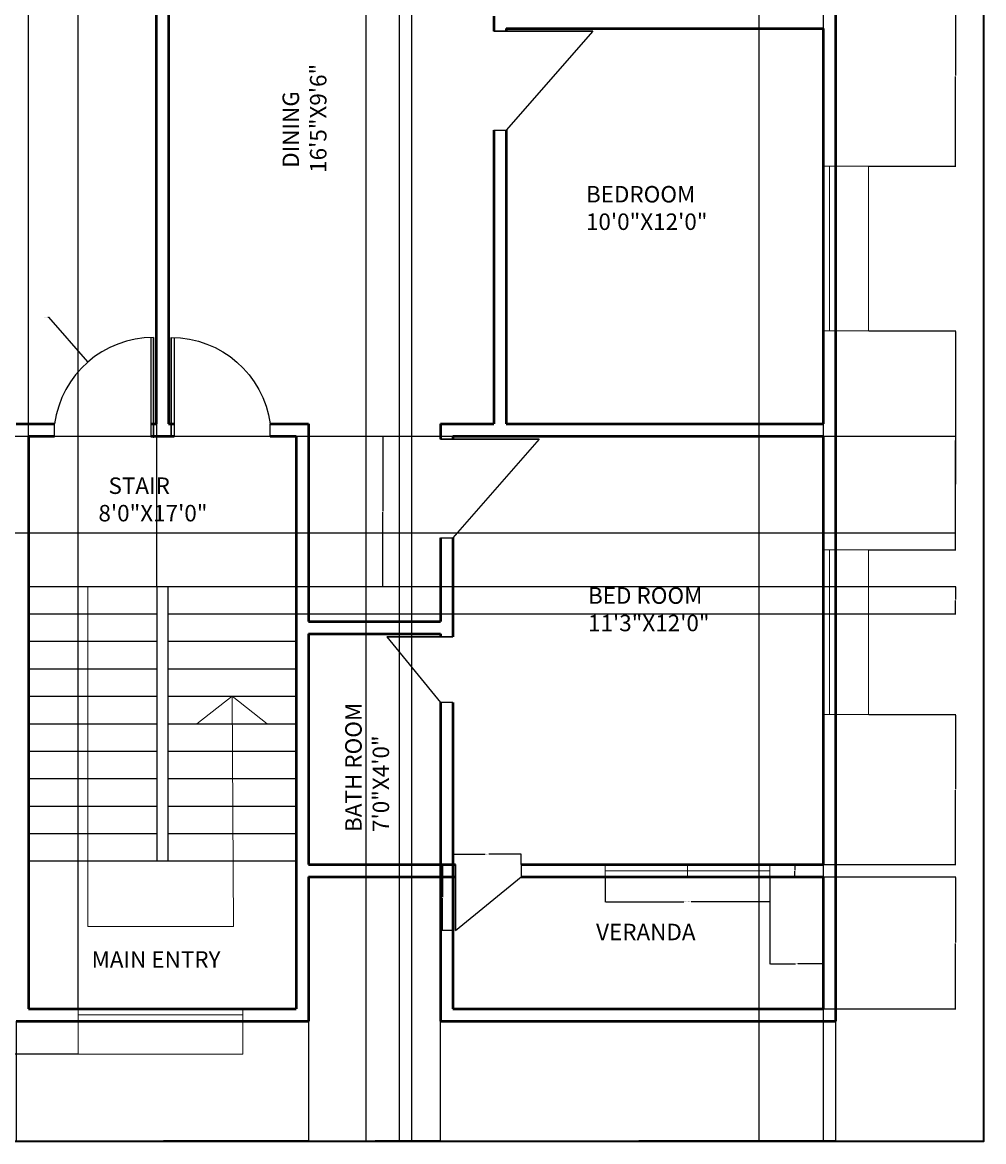
# Model space of a CAD drawing. Units: inches. Extents: x 2412 to 3014, y 10657 to 11360.
# Tile 2 of 3: x 2664 to 3014, y 10657 to 11065. Entities that reach past the tile are written whole.
import ezdxf

# ---------------------------------------------------------------- set-up
doc = ezdxf.new("R2010")
doc.units = ezdxf.units.IN
doc.header["$MEASUREMENT"] = 0
for name, color, linetype, lineweight in [('A-ANNO-DIMS', 2, 'Continuous', 18), ('A-ANNO-SYMB', 200, 'Continuous', 18), ('A-ANNO-TTLB', 7, 'Continuous', 35), ('A-AREA-IDEN', 7, 'Continuous', 18), ('A-DOOR', 22, 'Continuous', 25), ('A-FLOR-STRS', 200, 'Continuous', 25), ('A-GLAZ', 160, 'Continuous', 18), ('A-WALL', 142, 'Continuous', 50)]:
    doc.layers.add(name, color=color, linetype=linetype, lineweight=lineweight)
doc.styles.get("Standard").update_dxf_attribs({"font": 'arial.ttf'})
doc.dimstyles.get("Standard").update_dxf_attribs({"dimtxt": 0.18, "dimasz": 0.18, "dimexe": 0.18, "dimexo": 0.0625, "dimgap": 0.09, "dimtad": 0, "dimtih": 1, "dimtoh": 1, "dimdec": 4, "dimzin": 0, "dimdsep": 46, "dimtxsty": 'Standard', "dimcen": 0.09, "dimadec": 0, "dimazin": 0, "dimtfac": 1, "dimtdec": 4, "dimtofl": 0, "dimtmove": 0, "dimatfit": 3, "dimfxl": 1, "dimtolj": 1, "dimtzin": 0, "dimarcsym": 0})

# ---------------------------------------------------------------- blocks, each defined once
blk = doc.blocks.new('WIN-60IN-PROJECTING-SILL')
for p, q in [((0, 0), (0, 12)), ((0, 12), (60, 12)), ((60, 12), (60, 0)), ((0, 0), (0, -4.5)), ((60, 0), (0, 0)), ((60, -4.5), (60, 0)), ((60, -2.25), (0, -2.25)), ((0, -4.5), (60, -4.5))]:
    blk.add_line(p, q)
blk = doc.blocks.new('WIN-60IN-DIVIDED')
for p, q in [((0, 0), (0, -4.5)), ((60, 0), (0, 0)), ((30, 0), (30, -4.5)), ((60, -4.5), (60, 0)), ((0, -2.25), (60, -2.25)), ((0, -4.5), (60, -4.5))]:
    blk.add_line(p, q)
blk = doc.blocks.new('DOOR-36IN-ARC')
for p, q in [((-1, 36), (-1, 0)), ((0, 0), (0, 36)), ((0, 36), (0, 0)), ((-36, 0), (-36, 4.5)), ((0, 0), (-1, 0)), ((1, 0), (0, 0))]:
    blk.add_line(p, q)
blk.add_arc((0, -0.32), 36.32, 90, 172.3719)
blk = doc.blocks.new('DOOR-24IN-DIAGONAL')
for p, q in [((0, 24), (-24, 4.5)), ((0, 0), (0, 24)), ((0, 24), (0, 0)), ((-24, 0), (-24, 4.5)), ((1, 0), (0, 0))]:
    blk.add_line(p, q)
blk = doc.blocks.new('DOOR-36IN-DIAGONAL')
for p, q in [((0, 0), (-36, 0)), ((-36, 0), (0, 0)), ((-36, 0), (-4.5, -36)), ((0, 1), (0, 0)), ((0, -36), (-4.5, -36))]:
    blk.add_line(p, q)
blk = doc.blocks.new('*D10')
at = {"layer": 'A-ANNO-DIMS', "color": 0, "lineweight": -2, "transparency": 16777216}
for p, q in [((2876.44, 10753.72), (2876.44, 10744.6)), ((2936.44, 10753.72), (2936.44, 10744.6)), ((2876.62, 10744.78), (2905.1, 10744.78)), ((2936.26, 10744.78), (2907.78, 10744.78))]:
    blk.add_line(p, q, dxfattribs=at)
at = {"layer": 'A-ANNO-DIMS', "color": 0, "transparency": 16777216}
for points in [[(2876.62, 10744.81), (2876.62, 10744.75), (2876.44, 10744.78)], [(2936.26, 10744.81), (2936.26, 10744.75), (2936.44, 10744.78)]]:
    blk.add_solid(points, dxfattribs=at)
at = {"layer": 'Defpoints', "color": 0, "transparency": 16777216}
for p in [(2876.44, 10753.78), (2936.44, 10753.78), (2936.44, 10744.78)]:
    blk.add_point(p, dxfattribs=at)
at = {"layer": 'A-ANNO-DIMS', "color": 0, "transparency": 16777216, "insert": (2906.44, 10744.78), "char_height": 0.18, "attachment_point": 5}
blk.add_mtext('\\A1;WINDOW W2 60 TYP.', dxfattribs=at)
blk = doc.blocks.new('*D11')
at = {"layer": 'A-ANNO-DIMS', "color": 0, "lineweight": -2, "transparency": 16777216}
for p, q in [((2936.5, 10758.28), (2945.62, 10758.28)), ((2945.44, 10758.1), (2945.44, 10756.21)), ((2936.5, 10753.78), (2945.62, 10753.78)), ((2945.44, 10753.96), (2945.44, 10755.85))]:
    blk.add_line(p, q, dxfattribs=at)
at = {"layer": 'A-ANNO-DIMS', "color": 0, "transparency": 16777216}
for points in [[(2945.41, 10758.1), (2945.47, 10758.1), (2945.44, 10758.28)], [(2945.41, 10753.96), (2945.47, 10753.96), (2945.44, 10753.78)]]:
    blk.add_solid(points, dxfattribs=at)
at = {"layer": 'Defpoints', "color": 0, "transparency": 16777216}
for p in [(2936.44, 10758.28), (2945.44, 10758.28), (2936.44, 10753.78)]:
    blk.add_point(p, dxfattribs=at)
at = {"layer": 'A-ANNO-DIMS', "color": 0, "transparency": 16777216, "insert": (2945.44, 10756.03), "char_height": 0.18, "attachment_point": 5}
blk.add_mtext('\\A1;5 TYP.', dxfattribs=at)
blk = doc.blocks.new('*D20')
at = {"layer": 'A-ANNO-DIMS', "color": 0, "lineweight": -2, "transparency": 16777216}
for p, q in [((2820.86, 10758.34), (2820.86, 10762.21)), ((2821.04, 10762.03), (2832.64, 10762.03)), ((2845.68, 10762.03), (2834.08, 10762.03)), ((2845.86, 10758.34), (2845.86, 10762.21))]:
    blk.add_line(p, q, dxfattribs=at)
at = {"layer": 'A-ANNO-DIMS', "color": 0, "transparency": 16777216}
for points in [[(2821.04, 10762.06), (2821.04, 10762), (2820.86, 10762.03)], [(2845.68, 10762.06), (2845.68, 10762), (2845.86, 10762.03)]]:
    blk.add_solid(points, dxfattribs=at)
at = {"layer": 'Defpoints', "color": 0, "transparency": 16777216}
for p in [(2820.86, 10762.03), (2820.86, 10758.28), (2845.86, 10758.28)]:
    blk.add_point(p, dxfattribs=at)
at = {"layer": 'A-ANNO-DIMS', "color": 0, "transparency": 16777216, "insert": (2833.36, 10762.03), "char_height": 0.18, "attachment_point": 5}
blk.add_mtext('\\A1;D4 25 TYP.', dxfattribs=at)
blk = doc.blocks.new('*D21')
at = {"layer": 'A-ANNO-DIMS', "color": 0, "lineweight": -2, "transparency": 16777216}
for p, q in [((2820.8, 10758.28), (2816.93, 10758.28)), ((2817.11, 10758.1), (2817.11, 10746.46)), ((2817.11, 10734.46), (2817.11, 10746.1)), ((2820.8, 10734.28), (2816.93, 10734.28))]:
    blk.add_line(p, q, dxfattribs=at)
at = {"layer": 'A-ANNO-DIMS', "color": 0, "transparency": 16777216}
for points in [[(2817.08, 10758.1), (2817.14, 10758.1), (2817.11, 10758.28)], [(2817.08, 10734.46), (2817.14, 10734.46), (2817.11, 10734.28)]]:
    blk.add_solid(points, dxfattribs=at)
at = {"layer": 'Defpoints', "color": 0, "transparency": 16777216}
for p in [(2820.86, 10758.28), (2817.11, 10734.28), (2820.86, 10734.28)]:
    blk.add_point(p, dxfattribs=at)
at = {"layer": 'A-ANNO-DIMS', "color": 0, "transparency": 16777216, "insert": (2817.11, 10746.28), "char_height": 0.18, "attachment_point": 5}
blk.add_mtext('\\A1;24 TYP.', dxfattribs=at)
blk = doc.blocks.new('*D23')
at = {"layer": 'A-ANNO-DIMS', "color": 0, "lineweight": -2, "transparency": 16777216}
for p, q in [((2469.8, 11320.78), (2426.08, 11320.78)), ((2426.26, 11320.6), (2426.26, 11005.21)), ((2426.26, 10689.46), (2426.26, 11004.85)), ((2684.42, 10689.28), (2426.08, 10689.28))]:
    blk.add_line(p, q, dxfattribs=at)
at = {"layer": 'A-ANNO-DIMS', "color": 0, "transparency": 16777216}
for points in [[(2426.23, 11320.6), (2426.29, 11320.6), (2426.26, 11320.78)], [(2426.23, 10689.46), (2426.29, 10689.46), (2426.26, 10689.28)]]:
    blk.add_solid(points, dxfattribs=at)
at = {"layer": 'Defpoints', "color": 0, "transparency": 16777216}
for p in [(2426.26, 11320.78), (2469.86, 11320.78), (2684.48, 10689.28)]:
    blk.add_point(p, dxfattribs=at)
at = {"layer": 'A-ANNO-DIMS', "color": 0, "transparency": 16777216, "insert": (2426.26, 11005.03), "char_height": 0.18, "attachment_point": 5}
blk.add_mtext('\\A1;631.5', dxfattribs=at)
blk = doc.blocks.new('*D26')
at = {"layer": 'A-ANNO-DIMS', "color": 0, "lineweight": -2, "transparency": 16777216}
for p, q in [((2661.86, 10701.22), (2661.86, 10657.5)), ((2768.36, 10701.22), (2768.36, 10657.5)), ((2662.04, 10657.68), (2714.73, 10657.68)), ((2768.18, 10657.68), (2715.5, 10657.68))]:
    blk.add_line(p, q, dxfattribs=at)
at = {"layer": 'A-ANNO-DIMS', "color": 0, "transparency": 16777216}
for points in [[(2662.04, 10657.71), (2662.04, 10657.65), (2661.86, 10657.68)], [(2768.18, 10657.71), (2768.18, 10657.65), (2768.36, 10657.68)]]:
    blk.add_solid(points, dxfattribs=at)
at = {"layer": 'Defpoints', "color": 0, "transparency": 16777216}
for p in [(2661.86, 10701.28), (2768.36, 10701.28), (2768.36, 10657.68)]:
    blk.add_point(p, dxfattribs=at)
at = {"layer": 'A-ANNO-DIMS', "color": 0, "transparency": 16777216, "insert": (2715.11, 10657.68), "char_height": 0.18, "attachment_point": 5}
blk.add_mtext('\\A1;106.5', dxfattribs=at)
blk = doc.blocks.new('*D27')
at = {"layer": 'A-ANNO-DIMS', "color": 0, "lineweight": -2, "transparency": 16777216}
for p, q in [((2768.36, 10701.22), (2768.36, 10657.5)), ((2816.36, 10701.22), (2816.36, 10657.5)), ((2768.54, 10657.68), (2792.14, 10657.68)), ((2816.18, 10657.68), (2792.58, 10657.68))]:
    blk.add_line(p, q, dxfattribs=at)
at = {"layer": 'A-ANNO-DIMS', "color": 0, "transparency": 16777216}
for points in [[(2768.54, 10657.71), (2768.54, 10657.65), (2768.36, 10657.68)], [(2816.18, 10657.71), (2816.18, 10657.65), (2816.36, 10657.68)]]:
    blk.add_solid(points, dxfattribs=at)
at = {"layer": 'Defpoints', "color": 0, "transparency": 16777216}
for p in [(2768.36, 10701.28), (2816.36, 10701.28), (2816.36, 10657.68)]:
    blk.add_point(p, dxfattribs=at)
at = {"layer": 'A-ANNO-DIMS', "color": 0, "transparency": 16777216, "insert": (2792.36, 10657.68), "char_height": 0.18, "attachment_point": 5}
blk.add_mtext('\\A1;48', dxfattribs=at)
blk = doc.blocks.new('*D28')
at = {"layer": 'A-ANNO-DIMS', "color": 0, "lineweight": -2, "transparency": 16777216}
for p, q in [((2816.36, 10701.22), (2816.36, 10657.5)), ((2960.36, 10701.22), (2960.36, 10657.5)), ((2816.54, 10657.68), (2888.08, 10657.68)), ((2960.18, 10657.68), (2888.64, 10657.68))]:
    blk.add_line(p, q, dxfattribs=at)
at = {"layer": 'A-ANNO-DIMS', "color": 0, "transparency": 16777216}
for points in [[(2816.54, 10657.71), (2816.54, 10657.65), (2816.36, 10657.68)], [(2960.18, 10657.71), (2960.18, 10657.65), (2960.36, 10657.68)]]:
    blk.add_solid(points, dxfattribs=at)
at = {"layer": 'Defpoints', "color": 0, "transparency": 16777216}
for p in [(2816.36, 10701.28), (2960.36, 10701.28), (2960.36, 10657.68)]:
    blk.add_point(p, dxfattribs=at)
at = {"layer": 'A-ANNO-DIMS', "color": 0, "transparency": 16777216, "insert": (2888.36, 10657.68), "char_height": 0.18, "attachment_point": 5}
blk.add_mtext('\\A1;144', dxfattribs=at)
blk = doc.blocks.new('*D29')
at = {"layer": 'A-ANNO-DIMS', "color": 0, "lineweight": -2, "transparency": 16777216}
for p, q in [((2801.36, 11320.72), (2801.36, 10657.5)), ((2805.86, 11316.22), (2805.86, 10657.5)), ((2801.54, 10657.68), (2803.35, 10657.68)), ((2805.68, 10657.68), (2803.87, 10657.68))]:
    blk.add_line(p, q, dxfattribs=at)
at = {"layer": 'A-ANNO-DIMS', "color": 0, "transparency": 16777216}
for points in [[(2801.54, 10657.71), (2801.54, 10657.65), (2801.36, 10657.68)], [(2805.68, 10657.71), (2805.68, 10657.65), (2805.86, 10657.68)]]:
    blk.add_solid(points, dxfattribs=at)
at = {"layer": 'Defpoints', "color": 0, "transparency": 16777216}
for p in [(2801.36, 11320.78), (2805.86, 11316.28), (2805.86, 10657.68)]:
    blk.add_point(p, dxfattribs=at)
at = {"layer": 'A-ANNO-DIMS', "color": 0, "transparency": 16777216, "insert": (2803.61, 10657.68), "char_height": 0.18, "attachment_point": 5}
blk.add_mtext('\\A1;4.5', dxfattribs=at)
blk = doc.blocks.new('*D30')
at = {"layer": 'A-ANNO-DIMS', "color": 0, "lineweight": -2, "transparency": 16777216}
for p, q in [((2666.36, 10859.68), (2666.36, 11352.57)), ((2666.54, 11352.39), (2689.34, 11352.39)), ((2712.93, 11352.39), (2690.13, 11352.39)), ((2713.11, 10859.68), (2713.11, 11352.57))]:
    blk.add_line(p, q, dxfattribs=at)
at = {"layer": 'A-ANNO-DIMS', "color": 0, "transparency": 16777216}
for points in [[(2666.54, 11352.42), (2666.54, 11352.36), (2666.36, 11352.39)], [(2712.93, 11352.42), (2712.93, 11352.36), (2713.11, 11352.39)]]:
    blk.add_solid(points, dxfattribs=at)
at = {"layer": 'Defpoints', "color": 0, "transparency": 16777216}
for p in [(2713.11, 11352.39), (2666.36, 10859.62), (2713.11, 10859.62)]:
    blk.add_point(p, dxfattribs=at)
at = {"layer": 'A-ANNO-DIMS', "color": 0, "transparency": 16777216, "insert": (2689.74, 11352.39), "char_height": 0.18, "attachment_point": 5}
blk.add_mtext('\\A1;46.75', dxfattribs=at)
blk = doc.blocks.new('*D31')
at = {"layer": 'A-ANNO-DIMS', "color": 0, "lineweight": -2, "transparency": 16777216}
for p, q in [((2763.92, 10859.62), (3004.15, 10859.62)), ((3003.97, 10859.44), (3003.97, 10854.8)), ((3003.97, 10849.8), (3003.97, 10854.44)), ((2763.92, 10849.62), (3004.15, 10849.62))]:
    blk.add_line(p, q, dxfattribs=at)
at = {"layer": 'A-ANNO-DIMS', "color": 0, "transparency": 16777216}
for points in [[(3003.94, 10859.44), (3004, 10859.44), (3003.97, 10859.62)], [(3003.94, 10849.8), (3004, 10849.8), (3003.97, 10849.62)]]:
    blk.add_solid(points, dxfattribs=at)
at = {"layer": 'Defpoints', "color": 0, "transparency": 16777216}
for p in [(2763.86, 10859.62), (2763.86, 10849.62), (3003.97, 10849.62)]:
    blk.add_point(p, dxfattribs=at)
at = {"layer": 'A-ANNO-DIMS', "color": 0, "transparency": 16777216, "insert": (3003.97, 10854.62), "char_height": 0.18, "attachment_point": 5}
blk.add_mtext('\\A1;10', dxfattribs=at)
blk = doc.blocks.new('*D32')
at = {"layer": 'A-ANNO-DIMS', "color": 0, "lineweight": -2, "transparency": 16777216}
for p, q in [((2763.92, 10914.28), (2795.65, 10914.28)), ((2795.47, 10914.1), (2795.47, 10887.13)), ((2795.47, 10859.8), (2795.47, 10886.77)), ((2763.92, 10859.62), (2795.65, 10859.62))]:
    blk.add_line(p, q, dxfattribs=at)
at = {"layer": 'A-ANNO-DIMS', "color": 0, "transparency": 16777216}
for points in [[(2795.44, 10914.1), (2795.5, 10914.1), (2795.47, 10914.28)], [(2795.44, 10859.8), (2795.5, 10859.8), (2795.47, 10859.62)]]:
    blk.add_solid(points, dxfattribs=at)
at = {"layer": 'Defpoints', "color": 0, "transparency": 16777216}
for p in [(2763.86, 10914.28), (2763.86, 10859.62), (2795.47, 10859.62)]:
    blk.add_point(p, dxfattribs=at)
at = {"layer": 'A-ANNO-DIMS', "color": 0, "transparency": 16777216, "insert": (2795.47, 10886.95), "char_height": 0.18, "attachment_point": 5}
blk.add_mtext('\\A1;54.66', dxfattribs=at)
blk = doc.blocks.new('*D33')
at = {"layer": 'A-ANNO-DIMS', "color": 0, "lineweight": -2, "transparency": 16777216}
for p, q in [((2955.92, 10753.78), (3004.15, 10753.78)), ((3003.97, 10753.6), (3003.97, 10729.96)), ((3003.97, 10705.96), (3003.97, 10729.6)), ((2955.92, 10705.78), (3004.15, 10705.78))]:
    blk.add_line(p, q, dxfattribs=at)
at = {"layer": 'A-ANNO-DIMS', "color": 0, "transparency": 16777216}
for points in [[(3003.94, 10753.6), (3004, 10753.6), (3003.97, 10753.78)], [(3003.94, 10705.96), (3004, 10705.96), (3003.97, 10705.78)]]:
    blk.add_solid(points, dxfattribs=at)
at = {"layer": 'Defpoints', "color": 0, "transparency": 16777216}
for p in [(2955.86, 10753.78), (3003.97, 10753.78), (2955.86, 10705.78)]:
    blk.add_point(p, dxfattribs=at)
at = {"layer": 'A-ANNO-DIMS', "color": 0, "transparency": 16777216, "insert": (3003.97, 10729.78), "char_height": 0.18, "attachment_point": 5}
blk.add_mtext('\\A1;48', dxfattribs=at)
blk = doc.blocks.new('*D34')
at = {"layer": 'A-ANNO-DIMS', "color": 0, "lineweight": -2, "transparency": 16777216}
for p, q in [((2972.42, 10812.93), (3004.15, 10812.93)), ((3003.97, 10812.75), (3003.97, 10785.79)), ((3003.97, 10758.46), (3003.97, 10785.43)), ((2955.92, 10758.28), (3004.15, 10758.28))]:
    blk.add_line(p, q, dxfattribs=at)
at = {"layer": 'A-ANNO-DIMS', "color": 0, "transparency": 16777216}
for points in [[(3003.94, 10812.75), (3004, 10812.75), (3003.97, 10812.93)], [(3003.94, 10758.46), (3004, 10758.46), (3003.97, 10758.28)]]:
    blk.add_solid(points, dxfattribs=at)
at = {"layer": 'Defpoints', "color": 0, "transparency": 16777216}
for p in [(2972.36, 10812.93), (3003.97, 10812.93), (2955.86, 10758.28)]:
    blk.add_point(p, dxfattribs=at)
at = {"layer": 'A-ANNO-DIMS', "color": 0, "transparency": 16777216, "insert": (3003.97, 10785.61), "char_height": 0.18, "attachment_point": 5}
blk.add_mtext('\\A1;54.65', dxfattribs=at)
blk = doc.blocks.new('*D35')
at = {"layer": 'A-ANNO-DIMS', "color": 0, "lineweight": -2, "transparency": 16777216}
for p, q in [((2972.42, 10952.65), (3004.15, 10952.65)), ((3003.97, 10952.47), (3003.97, 10912.97)), ((3003.97, 10873.11), (3003.97, 10912.61)), ((2972.42, 10872.93), (3004.15, 10872.93))]:
    blk.add_line(p, q, dxfattribs=at)
at = {"layer": 'A-ANNO-DIMS', "color": 0, "transparency": 16777216}
for points in [[(3003.94, 10952.47), (3004, 10952.47), (3003.97, 10952.65)], [(3003.94, 10873.11), (3004, 10873.11), (3003.97, 10872.93)]]:
    blk.add_solid(points, dxfattribs=at)
at = {"layer": 'Defpoints', "color": 0, "transparency": 16777216}
for p in [(2972.36, 10952.65), (3003.97, 10952.65), (2972.36, 10872.93)]:
    blk.add_point(p, dxfattribs=at)
at = {"layer": 'A-ANNO-DIMS', "color": 0, "transparency": 16777216, "insert": (3003.97, 10912.79), "char_height": 0.18, "attachment_point": 5}
blk.add_mtext('\\A1;79.71', dxfattribs=at)
blk = doc.blocks.new('*D36')
at = {"layer": 'A-ANNO-DIMS', "color": 0, "lineweight": -2, "transparency": 16777216}
for p, q in [((2972.42, 11078.46), (3004.15, 11078.46)), ((3003.97, 11078.28), (3003.97, 11045.74)), ((3003.97, 11012.83), (3003.97, 11045.37)), ((2972.42, 11012.65), (3004.15, 11012.65))]:
    blk.add_line(p, q, dxfattribs=at)
at = {"layer": 'A-ANNO-DIMS', "color": 0, "transparency": 16777216}
for points in [[(3003.94, 11078.28), (3004, 11078.28), (3003.97, 11078.46)], [(3003.94, 11012.83), (3004, 11012.83), (3003.97, 11012.65)]]:
    blk.add_solid(points, dxfattribs=at)
at = {"layer": 'Defpoints', "color": 0, "transparency": 16777216}
for p in [(2972.36, 11078.46), (3003.97, 11078.46), (2972.36, 11012.65)]:
    blk.add_point(p, dxfattribs=at)
at = {"layer": 'A-ANNO-DIMS', "color": 0, "transparency": 16777216, "insert": (3003.97, 11045.55), "char_height": 0.18, "attachment_point": 5}
blk.add_mtext('\\A1;65.82', dxfattribs=at)
blk = doc.blocks.new('*D46')
at = {"layer": 'A-ANNO-DIMS', "color": 0, "lineweight": -2, "transparency": 16777216}
for p, q in [((2474.42, 10914.28), (3004.15, 10914.28)), ((3003.97, 10914.1), (3003.97, 10896.9)), ((3003.97, 10879.33), (3003.97, 10896.53)), ((2474.42, 10879.15), (3004.15, 10879.15))]:
    blk.add_line(p, q, dxfattribs=at)
at = {"layer": 'A-ANNO-DIMS', "color": 0, "transparency": 16777216}
for points in [[(3003.94, 10914.1), (3004, 10914.1), (3003.97, 10914.28)], [(3003.94, 10879.33), (3004, 10879.33), (3003.97, 10879.15)]]:
    blk.add_solid(points, dxfattribs=at)
at = {"layer": 'Defpoints', "color": 0, "transparency": 16777216}
for p in [(2474.36, 10914.28), (3003.97, 10914.28), (2474.36, 10879.15)]:
    blk.add_point(p, dxfattribs=at)
at = {"layer": 'A-ANNO-DIMS', "color": 0, "transparency": 16777216, "insert": (3003.97, 10896.71), "char_height": 0.18, "attachment_point": 5}
blk.add_mtext('\\A1;35.13', dxfattribs=at)
blk = doc.blocks.new('*D47')
at = {"layer": 'A-ANNO-DIMS', "color": 0, "lineweight": -2, "transparency": 16777216}
for p, q in [((2932.41, 11263.72), (2932.41, 10657.5)), ((2955.86, 11263.72), (2955.86, 10657.5)), ((2932.59, 10657.68), (2943.67, 10657.68)), ((2955.68, 10657.68), (2944.6, 10657.68))]:
    blk.add_line(p, q, dxfattribs=at)
at = {"layer": 'A-ANNO-DIMS', "color": 0, "transparency": 16777216}
for points in [[(2932.59, 10657.71), (2932.59, 10657.65), (2932.41, 10657.68)], [(2955.68, 10657.71), (2955.68, 10657.65), (2955.86, 10657.68)]]:
    blk.add_solid(points, dxfattribs=at)
at = {"layer": 'Defpoints', "color": 0, "transparency": 16777216}
for p in [(2932.41, 11263.78), (2955.86, 11263.78), (2955.86, 10657.68)]:
    blk.add_point(p, dxfattribs=at)
at = {"layer": 'A-ANNO-DIMS', "color": 0, "transparency": 16777216, "insert": (2944.13, 10657.68), "char_height": 0.18, "attachment_point": 5}
blk.add_mtext('\\A1;23.453', dxfattribs=at)
blk = doc.blocks.new('*D48')
at = {"layer": 'A-ANNO-DIMS', "color": 0, "lineweight": -2, "transparency": 16777216}
for p, q in [((2789.19, 11263.72), (2789.19, 10657.5)), ((2801.36, 11263.72), (2801.36, 10657.5)), ((2789.37, 10657.68), (2794.82, 10657.68)), ((2801.18, 10657.68), (2795.73, 10657.68))]:
    blk.add_line(p, q, dxfattribs=at)
at = {"layer": 'A-ANNO-DIMS', "color": 0, "transparency": 16777216}
for points in [[(2789.37, 10657.71), (2789.37, 10657.65), (2789.19, 10657.68)], [(2801.18, 10657.71), (2801.18, 10657.65), (2801.36, 10657.68)]]:
    blk.add_solid(points, dxfattribs=at)
at = {"layer": 'Defpoints', "color": 0, "transparency": 16777216}
for p in [(2789.19, 11263.78), (2801.36, 11263.78), (2801.36, 10657.68)]:
    blk.add_point(p, dxfattribs=at)
at = {"layer": 'A-ANNO-DIMS', "color": 0, "transparency": 16777216, "insert": (2795.28, 10657.68), "char_height": 0.18, "attachment_point": 5}
blk.add_mtext('\\A1;12.166', dxfattribs=at)
blk = doc.blocks.new('*D49')
at = {"layer": 'A-ANNO-DIMS', "color": 0, "lineweight": -2, "transparency": 16777216}
for p, q in [((2936.44, 10753.72), (2936.44, 10722)), ((2955.86, 10753.72), (2955.86, 10722)), ((2936.62, 10722.18), (2945.69, 10722.18)), ((2955.68, 10722.18), (2946.6, 10722.18))]:
    blk.add_line(p, q, dxfattribs=at)
at = {"layer": 'A-ANNO-DIMS', "color": 0, "transparency": 16777216}
for points in [[(2936.62, 10722.21), (2936.62, 10722.15), (2936.44, 10722.18)], [(2955.68, 10722.21), (2955.68, 10722.15), (2955.86, 10722.18)]]:
    blk.add_solid(points, dxfattribs=at)
at = {"layer": 'Defpoints', "color": 0, "transparency": 16777216}
for p in [(2936.44, 10753.78), (2955.86, 10753.78), (2936.44, 10722.18)]:
    blk.add_point(p, dxfattribs=at)
at = {"layer": 'A-ANNO-DIMS', "color": 0, "transparency": 16777216, "insert": (2946.15, 10722.18), "char_height": 0.18, "attachment_point": 5}
blk.add_mtext('\\A1;19.424', dxfattribs=at)
blk = doc.blocks.new('*D50')
at = {"layer": 'A-ANNO-DIMS', "color": 0, "lineweight": -2, "transparency": 16777216}
for p, q in [((2666.36, 10705.84), (2666.36, 11352.57)), ((2666.54, 11352.39), (2674.96, 11352.39)), ((2684.3, 11352.39), (2675.87, 11352.39)), ((2684.48, 10705.84), (2684.48, 11352.57))]:
    blk.add_line(p, q, dxfattribs=at)
at = {"layer": 'A-ANNO-DIMS', "color": 0, "transparency": 16777216}
for points in [[(2666.54, 11352.42), (2666.54, 11352.36), (2666.36, 11352.39)], [(2684.3, 11352.42), (2684.3, 11352.36), (2684.48, 11352.39)]]:
    blk.add_solid(points, dxfattribs=at)
at = {"layer": 'Defpoints', "color": 0, "transparency": 16777216}
for p in [(2684.48, 11352.39), (2666.36, 10705.78), (2684.48, 10705.78)]:
    blk.add_point(p, dxfattribs=at)
at = {"layer": 'A-ANNO-DIMS', "color": 0, "transparency": 16777216, "insert": (2675.42, 11352.39), "char_height": 0.18, "attachment_point": 5}
blk.add_mtext('\\A1;18.116', dxfattribs=at)
blk = doc.blocks.new('*D51')
at = {"layer": 'A-ANNO-DIMS', "color": 0, "lineweight": -2, "transparency": 16777216}
for p, q in [((2673.41, 10957.69), (2673.59, 10957.69)), ((2673.59, 10957.69), (2687.82, 10941.43)), ((2711.77, 10913.96), (2711.95, 10913.96)), ((2711.86, 10913.87), (2711.86, 10914.05))]:
    blk.add_line(p, q, dxfattribs=at)
at = {"layer": 'A-ANNO-DIMS', "color": 0, "transparency": 16777216}
blk.add_solid([(2687.85, 10941.45), (2687.8, 10941.41), (2687.94, 10941.29)], dxfattribs=at)
at = {"layer": 'Defpoints', "color": 0, "transparency": 16777216}
for p in [(2687.94, 10941.29), (2711.86, 10913.96)]:
    blk.add_point(p, dxfattribs=at)
at = {"layer": 'A-ANNO-DIMS', "color": 0, "transparency": 16777216, "insert": (2672.74, 10957.69), "char_height": 0.18, "attachment_point": 5}
blk.add_mtext('\\A1;4X R36.32', dxfattribs=at)

msp = doc.modelspace()

# ---------------------------------------------------------------- linework, layer by layer
at = {"layer": 'A-ANNO-SYMB'}
for p, q in [((2687.9507, 10859.6178), (2687.9507, 10735.7398)), ((2740.4863, 10819.6178), (2727.6399, 10809.6178)), ((2741.0291, 10735.7398), (2740.4863, 10819.6178)), ((2740.4863, 10819.6178), (2753.3327, 10809.6178)), ((2687.9507, 10735.7398), (2741.0291, 10735.7398))]:
    msp.add_line(p, q, dxfattribs=at)
at = {"layer": 'A-ANNO-TTLB'}
msp.add_lwpolyline([(2412.4885, 11360.4742), (3014.2671, 11360.4742), (3014.2671, 10657.3977), (2412.4885, 10657.3977)], close=True, dxfattribs=at)
at = {"layer": 'A-FLOR-STRS'}
for p, q in [((2666.3613, 10859.6178), (2763.8613, 10859.6178)), ((2713.1113, 10859.6178), (2713.1113, 10759.6178)), ((2717.1113, 10859.6178), (2717.1113, 10759.6178)), ((2666.3613, 10849.6178), (2713.1113, 10849.6178)), ((2717.1113, 10849.6178), (2763.8613, 10849.6178)), ((2666.3613, 10839.6178), (2713.1113, 10839.6178)), ((2717.1113, 10839.6178), (2763.8613, 10839.6178)), ((2666.3613, 10829.6178), (2713.1113, 10829.6178)), ((2717.1113, 10829.6178), (2763.8613, 10829.6178)), ((2666.3613, 10819.6178), (2713.1113, 10819.6178)), ((2717.1113, 10819.6178), (2763.8613, 10819.6178)), ((2666.3613, 10809.6178), (2713.1113, 10809.6178)), ((2717.1113, 10809.6178), (2763.8613, 10809.6178)), ((2666.3613, 10799.6178), (2713.1113, 10799.6178)), ((2717.1113, 10799.6178), (2763.8613, 10799.6178)), ((2666.3613, 10789.6178), (2713.1113, 10789.6178)), ((2717.1113, 10789.6178), (2763.8613, 10789.6178)), ((2666.3613, 10779.6178), (2713.1113, 10779.6178)), ((2717.1113, 10779.6178), (2763.8613, 10779.6178)), ((2666.3613, 10769.6178), (2713.1113, 10769.6178)), ((2717.1113, 10769.6178), (2763.8613, 10769.6178)), ((2666.3613, 10759.6178), (2763.8613, 10759.6178))]:
    msp.add_line(p, q, dxfattribs=at)
at = {"layer": 'A-WALL'}
for p, q in [((2960.3613, 11320.7803), (2960.3613, 10701.2803)), ((2712.8613, 11115.2803), (2712.8613, 10918.7803)), ((2717.3613, 11115.2803), (2717.3613, 10918.7803)), ((2835.8613, 11067.2803), (2835.8613, 11061.7803)), ((2840.3613, 11062.7803), (2840.3613, 11061.7803)), ((2840.3613, 11062.7803), (2955.8613, 11062.7803)), ((2955.8613, 11062.7803), (2955.8613, 10918.7803)), ((2835.8613, 11025.7803), (2835.8613, 10918.7803)), ((2840.3613, 11025.7803), (2840.3613, 10918.7803)), ((2661.8613, 10918.7803), (2675.8613, 10918.7803)), ((2710.8613, 10918.7803), (2712.8613, 10918.7803)), ((2717.3613, 10918.7803), (2719.3613, 10918.7803)), ((2754.3613, 10918.7803), (2768.3613, 10918.7803)), ((2768.3613, 10918.7803), (2768.3613, 10846.7803)), ((2816.3613, 10918.7803), (2816.3613, 10913.2803)), ((2816.3613, 10918.7803), (2835.8613, 10918.7803)), ((2840.3613, 10918.7803), (2955.8613, 10918.7803)), ((2666.3613, 10914.2803), (2666.3613, 10705.7803)), ((2666.3613, 10914.2803), (2675.8613, 10914.2803)), ((2710.8613, 10914.2803), (2719.3613, 10914.2803)), ((2754.3613, 10914.2803), (2763.8613, 10914.2803)), ((2763.8613, 10914.2803), (2763.8613, 10705.7803)), ((2820.8613, 10914.2803), (2820.8613, 10913.2803)), ((2820.8613, 10914.2803), (2955.8613, 10914.2803)), ((2955.8613, 10914.2803), (2955.8613, 10758.2803)), ((2816.3613, 10877.2803), (2816.3613, 10846.7803)), ((2820.8613, 10877.2803), (2820.8613, 10841.2803)), ((2768.3613, 10846.7803), (2816.3613, 10846.7803)), ((2768.3613, 10842.2803), (2816.3613, 10842.2803)), ((2768.3613, 10842.2803), (2768.3613, 10758.2803)), ((2816.3613, 10842.2803), (2816.3613, 10841.2803)), ((2816.3613, 10817.2803), (2816.3613, 10701.2803)), ((2820.8613, 10817.2803), (2820.8613, 10705.7803)), ((2768.3613, 10758.2803), (2821.8613, 10758.2803)), ((2845.8613, 10758.2803), (2955.8613, 10758.2803)), ((2768.3613, 10753.7803), (2821.8613, 10753.7803)), ((2768.3613, 10753.7803), (2768.3613, 10701.2803)), ((2845.8613, 10753.7803), (2955.8613, 10753.7803)), ((2955.8613, 10753.7803), (2955.8613, 10705.7803)), ((2666.3613, 10705.7803), (2763.8613, 10705.7803)), ((2820.8613, 10705.7803), (2955.8613, 10705.7803)), ((2661.8613, 10701.2803), (2768.3613, 10701.2803)), ((2816.3613, 10701.2803), (2960.3613, 10701.2803))]:
    msp.add_line(p, q, dxfattribs=at)

# ---------------------------------------------------------------- block references
at = {"layer": 'A-DOOR', "extrusion": (0, 0, -1), "zscale": -1}
for name, p in [('DOOR-36IN-DIAGONAL', (-2835.8613, 11061.7803)), ('DOOR-36IN-ARC', (-2718.3613, 10914.2803)), ('DOOR-36IN-DIAGONAL', (-2816.3613, 10913.2803))]:
    msp.add_blockref(name, p, dxfattribs=at)
at = {"layer": 'A-DOOR'}
msp.add_blockref('DOOR-36IN-ARC', (2711.8613, 10914.2803), dxfattribs=at)
for p, rotation in [((2820.8613, 10841.2803), 89.99999999998671), ((2821.8613, 10758.2803), 180)]:
    msp.add_blockref('DOOR-24IN-DIAGONAL', p, dxfattribs=dict(at, rotation=rotation))
at = {"layer": 'A-GLAZ'}
for p, rotation in [((2960.3613, 11012.6451), 270.0000000000108), ((2960.3613, 10872.9344), 270.0000000000153), ((2744.4775, 10701.2803), 180)]:
    msp.add_blockref('WIN-60IN-PROJECTING-SILL', p, dxfattribs=dict(at, rotation=rotation))
msp.add_blockref('WIN-60IN-DIVIDED', (2876.4377, 10758.2803), dxfattribs=at)

# ---------------------------------------------------------------- texts
at = {"layer": 'A-AREA-IDEN', "char_height": 6, "attachment_point": 1, "rotation": 90}
for s, width, insert in [(' DINING\\P16\'5"X9\'6"', 72.937811, (2758.888, 11010.2232)), ('BATH ROOM\\P7\'0"X4\'0"', 111.272779, (2781.7137, 10770.166))]:
    msp.add_mtext_dynamic_manual_height_columns(s, width=width, gutter_width=30, heights=[0], dxfattribs=dict(at, insert=insert))
at = {"layer": 'A-AREA-IDEN', "char_height": 6, "attachment_point": 1}
for s, width, heights, insert in [('BEDROOM\\P10\'0"X12\'0"', 65.951062, [0], (2869.4087, 11005.4406)), ('  STAIR\\P8\'0"X17\'0"', 51.386437, [0], (2691.8148, 10899.2871)), ('BED ROOM\\P11\'3"X12\'0"', 65.606634, [0], (2870.1646, 10859.2818)), ('VERANDA', 60.155979, [6], (2873.1007, 10736.7406)), ('MAIN ENTRY', 54.612409, [0], (2689.3214, 10726.7396))]:
    msp.add_mtext_dynamic_manual_height_columns(s, width=width, gutter_width=30, heights=heights, dxfattribs=dict(at, insert=insert))

# ---------------------------------------------------------------- dimensions: what is measured, and where the dimension line sits
at = {"layer": 'A-ANNO-DIMS'}
for base, p1, p2, override, picture, middle in [((2713.1113, 11352.3853), (2666.3613, 10859.6178), (2713.1113, 10859.6178), {"dimdec": 2, "dimlfac": 1, "dimrnd": 0, "dimzin": 0, "dimdsep": 46, "dimlunit": 2}, '*D30', (2689.7363, 11352.3853)), ((2684.4775, 11352.3853), (2666.3613, 10705.7803), (2684.4775, 10705.7803), {"dimdec": 3, "dimlfac": 1, "dimrnd": 0, "dimzin": 0, "dimdsep": 46, "dimlunit": 2}, '*D50', (2675.4194, 11352.3853)), ((2805.8613, 10657.6753), (2801.3613, 11320.7803), (2805.8613, 11316.2803), {"dimdec": 1, "dimlfac": 1, "dimrnd": 0, "dimzin": 0, "dimdsep": 46, "dimlunit": 2}, '*D29', (2803.6113, 10657.6753)), ((2801.3613, 10657.6753), (2789.195, 11263.7803), (2801.3613, 11263.7803), {"dimdec": 3, "dimlfac": 1, "dimrnd": 0, "dimzin": 0, "dimdsep": 46, "dimlunit": 2}, '*D48', (2795.2781, 10657.6753)), ((2955.8613, 10657.6753), (2932.4085, 11263.7803), (2955.8613, 11263.7803), {"dimdec": 3, "dimlfac": 1, "dimrnd": 0, "dimzin": 0, "dimdsep": 46, "dimlunit": 2}, '*D47', (2944.1349, 10657.6753)), ((2768.3613, 10657.6753), (2661.8613, 10701.2803), (2768.3613, 10701.2803), {"dimdec": 1, "dimlfac": 1, "dimrnd": 0, "dimzin": 0, "dimdsep": 46, "dimlunit": 2}, '*D26', (2715.1113, 10657.6753)), ((2816.3613, 10657.6753), (2768.3613, 10701.2803), (2816.3613, 10701.2803), {"dimdec": 0, "dimlfac": 1, "dimrnd": 0, "dimzin": 0, "dimdsep": 46, "dimlunit": 2}, '*D27', (2792.3613, 10657.6753)), ((2960.3613, 10657.6753), (2816.3613, 10701.2803), (2960.3613, 10701.2803), {"dimdec": 0, "dimlfac": 1, "dimrnd": 0, "dimzin": 0, "dimdsep": 46, "dimlunit": 2}, '*D28', (2888.3613, 10657.6753))]:
    dim = msp.add_linear_dim(base=base, p1=p1, p2=p2, dimstyle='Standard', override=override, dxfattribs=at)
    dim.commit()
    dim.dimension.update_dxf_attribs({"geometry": picture, "text_midpoint": middle})
for base, p1, p2, angle, override, picture, middle in [((2426.2563, 11320.7803), (2684.4775, 10689.2803), (2469.8613, 11320.7803), 90, {"dimdec": 1, "dimlfac": 1, "dimrnd": 0, "dimzin": 0, "dimdsep": 46, "dimlunit": 2}, '*D23', (2426.2563, 11005.0303)), ((3003.9663, 11078.4623), (2972.3613, 11012.6451), (2972.3613, 11078.4623), 90, {"dimdec": 2, "dimlfac": 1, "dimrnd": 0, "dimzin": 0, "dimdsep": 46, "dimlunit": 2}, '*D36', (3003.9663, 11045.5537)), ((3003.9663, 10952.6451), (2972.3613, 10872.9344), (2972.3613, 10952.6451), 90, {"dimdec": 2, "dimlfac": 1, "dimrnd": 0, "dimzin": 0, "dimdsep": 46, "dimlunit": 2}, '*D35', (3003.9663, 10912.7897)), ((3003.9663, 10914.2803), (2474.3613, 10879.149), (2474.3613, 10914.2803), 90, {"dimdec": 2, "dimlfac": 1, "dimrnd": 0, "dimzin": 0, "dimdsep": 46, "dimlunit": 2}, '*D46', (3003.9663, 10896.7146)), ((2795.4663, 10859.6178), (2763.8613, 10914.2803), (2763.8613, 10859.6178), 270, {"dimdec": 2, "dimlfac": 1, "dimrnd": 0, "dimzin": 0, "dimdsep": 46, "dimlunit": 2}, '*D32', (2795.4663, 10886.949)), ((3003.9663, 10849.6178), (2763.8613, 10859.6178), (2763.8613, 10849.6178), 90, {"dimdec": 0, "dimlfac": 1, "dimrnd": 0, "dimzin": 0, "dimdsep": 46, "dimlunit": 2}, '*D31', (3003.9663, 10854.6178)), ((3003.9663, 10812.9344), (2955.8613, 10758.2803), (2972.3613, 10812.9344), 90, {"dimdec": 2, "dimlfac": 1, "dimrnd": 0, "dimzin": 0, "dimdsep": 46, "dimlunit": 2}, '*D34', (3003.9663, 10785.6073)), ((2936.4377, 10722.1753), (2955.8613, 10753.7803), (2936.4377, 10753.7803), 180, {"dimdec": 3, "dimlfac": 1, "dimrnd": 0, "dimzin": 0, "dimdsep": 46, "dimlunit": 2}, '*D49', (2946.1495, 10722.1753)), ((3003.9663, 10753.7803), (2955.8613, 10705.7803), (2955.8613, 10753.7803), 90, {"dimdec": 0, "dimlfac": 1, "dimrnd": 0, "dimzin": 0, "dimdsep": 46, "dimlunit": 2}, '*D33', (3003.9663, 10729.7803))]:
    dim = msp.add_linear_dim(base=base, p1=p1, p2=p2, angle=angle, dimstyle='Standard', override=override, dxfattribs=at)
    dim.commit()
    dim.dimension.update_dxf_attribs({"geometry": picture, "text_midpoint": middle})
dim = msp.add_radius_dim(center=(2711.8613, 10913.9588), mpoint=(2687.9435, 10941.2935), text='4X <>', dimstyle='Standard', override={"dimdec": 2, "dimlfac": 1, "dimrnd": 0, "dimzin": 0, "dimdsep": 46, "dimlunit": 2}, dxfattribs=at)
dim.commit()
dim.dimension.update_dxf_attribs({"geometry": '*D51', "text_midpoint": (2672.7368, 10957.6943), "dimtype": 164})
for base, p1, p2, angle, text, picture, middle in [((2820.8613, 10762.0303), (2845.8613, 10758.2803), (2820.8613, 10758.2803), 180, 'D4 <> TYP.', '*D20', (2833.3613, 10762.0303)), ((2817.1113, 10734.2803), (2820.8613, 10758.2803), (2820.8613, 10734.2803), 270, '<> TYP.', '*D21', (2817.1113, 10746.2803)), ((2945.4376764996, 10758.2802714264), (2936.4376764996, 10753.7802714264), (2936.4376764996, 10758.2802714264), 90, '<> TYP.', '*D11', (2945.4376764996, 10756.0302714264))]:
    dim = msp.add_linear_dim(base=base, p1=p1, p2=p2, angle=angle, text=text, dimstyle='Standard', override={"dimdec": 0, "dimlfac": 1, "dimrnd": 0, "dimzin": 0, "dimdsep": 46, "dimlunit": 2}, dxfattribs=at)
    dim.commit()
    dim.dimension.update_dxf_attribs({"geometry": picture, "text_midpoint": middle})
dim = msp.add_linear_dim(base=(2936.4377, 10744.7803), p1=(2876.4377, 10753.7803), p2=(2936.4377, 10753.7803), text='WINDOW W2 <> TYP.', dimstyle='Standard', override={"dimdec": 0, "dimlfac": 1, "dimrnd": 0, "dimzin": 0, "dimdsep": 46, "dimlunit": 2}, dxfattribs=at)
dim.commit()
dim.dimension.update_dxf_attribs({"geometry": '*D10', "text_midpoint": (2906.4377, 10744.7803)})

doc.saveas('drawing.dxf')
